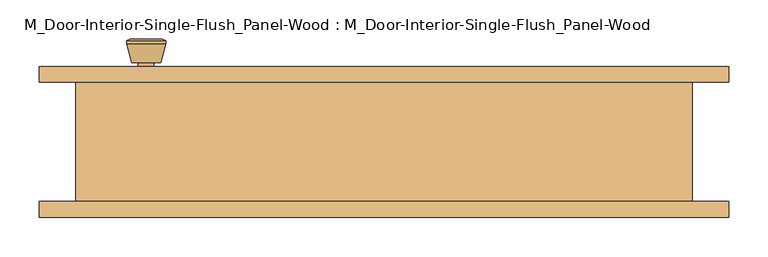
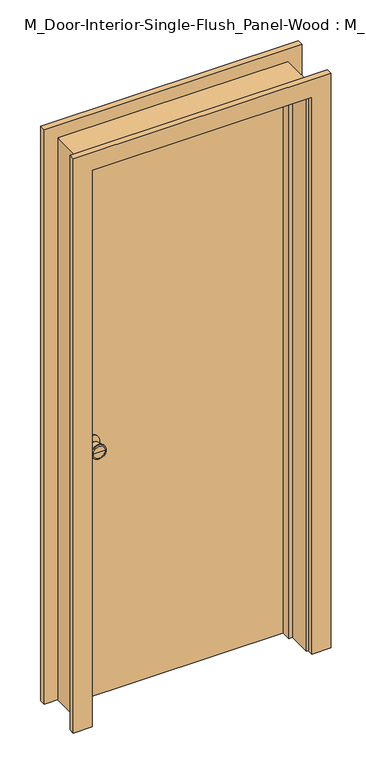
"""IFC4 building model written with IfcOpenShell, lengths in millimetres: door geometry, M_Door-Interior-Single-Flush_Panel-Wood : M_Door-Interior-Single-Flush_Panel-Wood."""

from ifc_helpers import new_model, si_unit, point, frame, frame_2d, origin, origin_with_axes, place, context, project, spatial, polyline, circle_curve, trimmed, segment, composite_curve, outline, extrude, faceted_brep, source, transform, mapped, element, save
from ifc_brep_helpers import plane_surface, cylinder_surface, revolved_surface, advanced_brep


def m_door_interior_single_flush_panel_wood_m_door_interior_da0777dc(model_context):
    return source(origin(), model_context, "Body", "SolidModel", [
        advanced_brep(
        [(-303.3, 32.025, 914.4), (-293.3, 32.025, 914.4), (-313.3, 32.025, 914.4), (-282.8241324, -16.975, 914.4), (-303.3, -16.975, 914.4), (-323.7758676, -16.975, 914.4), (-278.3, -15.1471319, 914.4), (-328.3, -15.1471319, 914.4), (-278.3, -11.6834537, 914.4), (-328.3, -11.6834537, 914.4), (-284.663764, 13.025, 914.4), (-321.936236, 13.025, 914.4), (-293.3, 13.025, 914.4), (-313.3, 13.025, 914.4)],
        [
            (0, 1),
            (1, 2, circle_curve(frame((-303.3, 32.025, 914.4), z_axis=(0.0, 1.0, 0.0), x_axis=(-1.0, 0.0, 0.0)), 10.0)),
            (2, 0),
            (2, 1, circle_curve(frame((-303.3, 32.025, 914.4), z_axis=(0.0, 1.0, 0.0), x_axis=(-1.0, 0.0, 0.0)), 10.0)),
            (3, 4),
            (4, 5),
            (5, 3, circle_curve(frame((-303.3, -16.975, 914.4), z_axis=(0.0, -1.0, 0.0), x_axis=(-1.0, 0.0, 0.0)), 20.4758676)),
            (3, 5, circle_curve(frame((-303.3, -16.975, 914.4), z_axis=(0.0, -1.0, 0.0), x_axis=(-1.0, 0.0, 0.0)), 20.4758676)),
            (6, 3),
            (5, 7),
            (7, 6, circle_curve(frame((-303.3, -15.1471319, 914.4), z_axis=(0.0, -1.0, 0.0), x_axis=(-1.0, 0.0, 0.0)), 25.0)),
            (6, 7, circle_curve(frame((-303.3, -15.1471319, 914.4), z_axis=(0.0, -1.0, 0.0), x_axis=(-1.0, 0.0, 0.0)), 25.0)),
            (8, 6),
            (7, 9),
            (9, 8, circle_curve(frame((-303.3, -11.6834537, 914.4), z_axis=(0.0, -1.0, 0.0), x_axis=(-1.0, 0.0, 0.0)), 25.0)),
            (8, 9, circle_curve(frame((-303.3, -11.6834537, 914.4), z_axis=(0.0, -1.0, 0.0), x_axis=(-1.0, 0.0, 0.0)), 25.0)),
            (10, 8),
            (9, 11),
            (11, 10, circle_curve(frame((-303.3, 13.025, 914.4), z_axis=(0.0, -1.0, 0.0), x_axis=(-1.0, 0.0, 0.0)), 18.636236)),
            (10, 11, circle_curve(frame((-303.3, 13.025, 914.4), z_axis=(0.0, -1.0, 0.0), x_axis=(-1.0, 0.0, 0.0)), 18.636236)),
            (12, 10),
            (11, 13),
            (13, 12, circle_curve(frame((-303.3, 13.025, 914.4), z_axis=(0.0, -1.0, 0.0), x_axis=(-1.0, 0.0, 0.0)), 10.0)),
            (12, 13, circle_curve(frame((-303.3, 13.025, 914.4), z_axis=(0.0, -1.0, 0.0), x_axis=(-1.0, 0.0, 0.0)), 10.0)),
            (1, 12),
            (13, 2),
        ],
        [
            plane_surface(frame((-303.3, 32.025, 914.4), z_axis=(0.0, 1.0, 0.0), x_axis=(-1.0, 0.0, 0.0))),
            plane_surface(frame((-303.3, -16.975, 914.4), z_axis=(0.0, -1.0, 0.0), x_axis=(-1.0, 0.0, 0.0))),
            revolved_surface(polyline([(-323.7758676, -16.975, 914.4), (-328.3, -15.1471319, 914.4)]), (-303.3, 32.025, 914.4), (0.0, 1.0, 0.0)),
            cylinder_surface(frame((-303.3, 32.025, 914.4), z_axis=(0.0, 1.0, 0.0), x_axis=(-1.0, 0.0, 0.0)), 25.0),
            revolved_surface(polyline([(-328.3, -11.6834537, 914.4), (-321.936236, 13.025, 914.4)]), (-303.3, 32.025, 914.4), (0.0, 1.0, 0.0)),
            plane_surface(frame((-303.3, 13.025, 914.4), z_axis=(0.0, 1.0, 0.0), x_axis=(-1.0, 0.0, 0.0))),
            cylinder_surface(frame((-303.3, 32.025, 914.4), z_axis=(0.0, 1.0, 0.0), x_axis=(-1.0, 0.0, 0.0)), 10.0),
        ],
        [
            (0, [[1, 2, 3]]),
            (0, [[-3, 4, -1]]),
            (1, [[5, 6, 7]]),
            (1, [[-6, -5, 8]]),
            (2, [[9, -7, 10, 11]]),
            (2, [[-10, -8, -9, 12]]),
            (3, [[13, -11, 14, 15]]),
            (3, [[-14, -12, -13, 16]]),
            (4, [[17, -15, 18, 19]]),
            (4, [[-18, -16, -17, 20]]),
            (5, [[21, -19, 22, 23]]),
            (5, [[-22, -20, -21, 24]]),
            (6, [[25, -23, 26, -2]]),
            (6, [[-26, -24, -25, -4]]),
        ],
    ),
        extrude(outline(composite_curve([segment(trimmed(circle_curve(frame_2d((914.4, -303.3)), 30.0), [point((914.4, -333.3))], [point((914.4, -273.3))], False, "CARTESIAN"), True, "CONTINUOUS"), segment(trimmed(circle_curve(frame_2d((914.4, -303.3)), 30.0), [point((914.4, -273.3))], [point((914.4, -333.3))], False, "CARTESIAN"), True, "CONTINUOUS")], self_intersect=False)), frame((0.0, 32.025, 0.0), z_axis=(0.0, 1.0, 0.0), x_axis=(0.0, 0.0, 1.0)), (0.0, 0.0, 1.0), 6.0),
        advanced_brep(
        [(-303.3, 79.025, 914.4), (-313.3, 79.025, 914.4), (-293.3, 79.025, 914.4), (-282.8241324, 128.025, 914.4), (-323.7758676, 128.025, 914.4), (-303.3, 128.025, 914.4), (-278.3, 126.1971319, 914.4), (-328.3, 126.1971319, 914.4), (-278.3, 122.7334537, 914.4), (-328.3, 122.7334537, 914.4), (-284.663764, 98.025, 914.4), (-321.936236, 98.025, 914.4), (-293.3, 98.025, 914.4), (-313.3, 98.025, 914.4)],
        [
            (0, 1),
            (1, 2, circle_curve(frame((-303.3, 79.025, 914.4), z_axis=(0.0, -1.0, 0.0), x_axis=(-1.0, 0.0, 0.0)), 10.0)),
            (2, 0),
            (2, 1, circle_curve(frame((-303.3, 79.025, 914.4), z_axis=(0.0, -1.0, 0.0), x_axis=(-1.0, 0.0, 0.0)), 10.0)),
            (3, 4, circle_curve(frame((-303.3, 128.025, 914.4), z_axis=(0.0, 1.0, 0.0), x_axis=(-1.0, 0.0, 0.0)), 20.4758676)),
            (4, 5),
            (5, 3),
            (4, 3, circle_curve(frame((-303.3, 128.025, 914.4), z_axis=(0.0, 1.0, 0.0), x_axis=(-1.0, 0.0, 0.0)), 20.4758676)),
            (6, 7, circle_curve(frame((-303.3, 126.1971319, 914.4), z_axis=(0.0, 1.0, 0.0), x_axis=(-1.0, 0.0, 0.0)), 25.0)),
            (7, 4),
            (3, 6),
            (7, 6, circle_curve(frame((-303.3, 126.1971319, 914.4), z_axis=(0.0, 1.0, 0.0), x_axis=(-1.0, 0.0, 0.0)), 25.0)),
            (8, 9, circle_curve(frame((-303.3, 122.7334537, 914.4), z_axis=(0.0, 1.0, 0.0), x_axis=(-1.0, 0.0, 0.0)), 25.0)),
            (9, 7),
            (6, 8),
            (9, 8, circle_curve(frame((-303.3, 122.7334537, 914.4), z_axis=(0.0, 1.0, 0.0), x_axis=(-1.0, 0.0, 0.0)), 25.0)),
            (10, 11, circle_curve(frame((-303.3, 98.025, 914.4), z_axis=(0.0, 1.0, 0.0), x_axis=(-1.0, 0.0, 0.0)), 18.636236)),
            (11, 9),
            (8, 10),
            (11, 10, circle_curve(frame((-303.3, 98.025, 914.4), z_axis=(0.0, 1.0, 0.0), x_axis=(-1.0, 0.0, 0.0)), 18.636236)),
            (12, 13, circle_curve(frame((-303.3, 98.025, 914.4), z_axis=(0.0, 1.0, 0.0), x_axis=(-1.0, 0.0, 0.0)), 10.0)),
            (13, 11),
            (10, 12),
            (13, 12, circle_curve(frame((-303.3, 98.025, 914.4), z_axis=(0.0, 1.0, 0.0), x_axis=(-1.0, 0.0, 0.0)), 10.0)),
            (1, 13),
            (12, 2),
        ],
        [
            plane_surface(frame((-303.3, 79.025, 914.4), z_axis=(0.0, -1.0, 0.0), x_axis=(-1.0, 0.0, 0.0))),
            plane_surface(frame((-303.3, 128.025, 914.4), z_axis=(0.0, 1.0, 0.0), x_axis=(-1.0, 0.0, 0.0))),
            revolved_surface(polyline([(-323.7758676, 128.025, 914.4), (-328.3, 126.1971319, 914.4)]), (-303.3, 79.025, 914.4), (0.0, -1.0, 0.0)),
            cylinder_surface(frame((-303.3, 79.025, 914.4), z_axis=(0.0, -1.0, 0.0), x_axis=(-1.0, 0.0, 0.0)), 25.0),
            revolved_surface(polyline([(-328.3, 122.7334537, 914.4), (-321.936236, 98.025, 914.4)]), (-303.3, 79.025, 914.4), (0.0, -1.0, 0.0)),
            plane_surface(frame((-303.3, 98.025, 914.4), z_axis=(0.0, -1.0, 0.0), x_axis=(-1.0, 0.0, 0.0))),
            cylinder_surface(frame((-303.3, 79.025, 914.4), z_axis=(0.0, -1.0, 0.0), x_axis=(-1.0, 0.0, 0.0)), 10.0),
        ],
        [
            (0, [[1, 2, 3]]),
            (0, [[-3, 4, -1]]),
            (1, [[5, 6, 7]]),
            (1, [[8, -7, -6]]),
            (2, [[9, 10, -5, 11]]),
            (2, [[12, -11, -8, -10]]),
            (3, [[13, 14, -9, 15]]),
            (3, [[16, -15, -12, -14]]),
            (4, [[17, 18, -13, 19]]),
            (4, [[20, -19, -16, -18]]),
            (5, [[21, 22, -17, 23]]),
            (5, [[24, -23, -20, -22]]),
            (6, [[-2, 25, -21, 26]]),
            (6, [[-4, -26, -24, -25]]),
        ],
    ),
        extrude(outline(composite_curve([segment(trimmed(circle_curve(frame_2d((914.4, -303.3)), 30.0), [point((914.4, -333.3))], [point((914.4, -273.3))], False, "CARTESIAN"), True, "CONTINUOUS"), segment(trimmed(circle_curve(frame_2d((914.4, -303.3)), 30.0), [point((914.4, -273.3))], [point((914.4, -333.3))], False, "CARTESIAN"), True, "CONTINUOUS")], self_intersect=False)), frame((0.0, 73.025, 0.0), z_axis=(0.0, 1.0, 0.0), x_axis=(0.0, 0.0, 1.0)), (0.0, 0.0, 1.0), 6.0),
        faceted_brep([(393.3, 73.025, 0.0), (393.3, -79.375, 0.0), (368.3, -79.375, 0.0), (368.3, 3.1, 0.0), (355.6, 3.1, 0.0), (355.6, 38.025, 0.0), (368.3, 38.025, 0.0), (368.3, 73.025, 0.0), (393.3, 73.025, 2025.0), (393.3, -79.375, 2025.0), (-393.3, -79.375, 2025.0), (-393.3, -79.375, 0.0), (-368.3, -79.375, 0.0), (-368.3, -79.375, 2000.0), (368.3, -79.375, 2000.0), (368.3, 3.1, 2000.0), (-368.3, 3.1, 2000.0), (-368.3, 3.1, 0.0), (-355.6, 3.1, 0.0), (-355.6, 3.1, 1987.3), (355.6, 3.1, 1987.3), (355.6, 38.025, 1987.3), (-355.6, 38.025, 1987.3), (-355.6, 38.025, 0.0), (-368.3, 38.025, 0.0), (-368.3, 38.025, 2000.0), (368.3, 38.025, 2000.0), (368.3, 73.025, 2000.0), (-368.3, 73.025, 2000.0), (-368.3, 73.025, 0.0), (-393.3, 73.025, 0.0), (-393.3, 73.025, 2025.0)], [[[0, 1, 2, 3, 4, 5, 6, 7]], [[1, 0, 8, 9]], [[2, 1, 9, 10, 11, 12, 13, 14]], [[3, 2, 14, 15]], [[4, 3, 15, 16, 17, 18, 19, 20]], [[5, 4, 20, 21]], [[6, 5, 21, 22, 23, 24, 25, 26]], [[7, 6, 26, 27]], [[0, 7, 27, 28, 29, 30, 31, 8]], [[9, 8, 31, 10]], [[15, 14, 13, 16]], [[21, 20, 19, 22]], [[27, 26, 25, 28]], [[30, 29, 24, 23, 18, 17, 12, 11]], [[10, 31, 30, 11]], [[16, 13, 12, 17]], [[22, 19, 18, 23]], [[28, 25, 24, 29]]]),
        extrude(outline(polyline([(368.3, 38.025), (-368.3, 38.025), (-368.3, 73.025), (368.3, 73.025), (368.3, 38.025)])), origin_with_axes(), (0.0, 0.0, 1.0), 2000.0),
        extrude(outline(polyline([(0.0, 374.65), (0.0, 439.65), (2071.35, 439.65), (2071.35, -439.65), (0.0, -439.65), (0.0, -374.65), (2006.35, -374.65), (2006.35, 374.65), (0.0, 374.65)])), frame((0.0, 73.025, 0.0), z_axis=(0.0, 1.0, 0.0), x_axis=(0.0, 0.0, 1.0)), (0.0, 0.0, 1.0), 20.0),
        extrude(outline(polyline([(0.0, 374.65), (0.0, 439.65), (2071.35, 439.65), (2071.35, -439.65), (0.0, -439.65), (0.0, -374.65), (2006.35, -374.65), (2006.35, 374.65), (0.0, 374.65)])), frame((0.0, -99.375, 0.0), z_axis=(0.0, 1.0, 0.0), x_axis=(0.0, 0.0, 1.0)), (0.0, 0.0, 1.0), 20.0),
    ])


if __name__ == "__main__":
    model = new_model("IFC4")
    model_context = context("Model", 3, world=origin())
    ifc_project = project(units=[si_unit("LENGTHUNIT", "METRE", prefix="MILLI")], contexts=[model_context])
    site = spatial("IfcSite", under=ifc_project)
    building = spatial("IfcBuilding", under=site)
    placement = place(None, origin())
    m_door_interior_single_flush_panel_wood_m_door_interior_shape = m_door_interior_single_flush_panel_wood_m_door_interior_da0777dc(model_context)
    element("IfcDoor", 1, ObjectType="M_Door-Interior-Single-Flush_Panel-Wood : M_Door-Interior-Single-Flush_Panel-Wood", at=placement, inside=building, context=model_context, shape_type="MappedRepresentation", body=[
        mapped(m_door_interior_single_flush_panel_wood_m_door_interior_shape, transform((0.0, 0.0, 0.0), x_axis=(1.0, 0.0, 0.0), y_axis=(0.0, 1.0, 0.0), z_axis=(0.0, 0.0, 1.0))),
    ])
    save(model, "model.ifc")

# Revit data of these elements
# Type "M_Door-Interior-Single-Flush_Panel-Wood : M_Door-Interior-Single-Flush_Panel-Wood"
#   Type Mark = "10"
#   Assembly Code = "C1020300"
#   Analytic Construction = "Wooden"
#   Thickness = 0' - 1.37795"
#   Thermal Resistance (R) = 2.5876 (h·ft²·°F)/BTU
#   Swing Angle [instance default] = 90.00°
#   Rough Width = 2' - 6.9685"
#   Rough Height = 6' - 7.72441"
#   Height = 6' - 6.74016"
#   Width = 2' - 5"
#   Heat Transfer Coefficient (U) = 0.3865 BTU/(h·ft²·°F)
#   Trim Material = Cherry
#   Panel Material = Cherry
#   Frame Material = Cherry
#   Door Handle Material = Aluminum
#   Visual Light Transmittance = 0
#   Solar Heat Gain Coefficient = 0
#   Wall Closure = (empty or 0)
#   Function = (empty or 0)
# Element 1 (IfcDoor, "M_Door-Interior-Single-Flush_Panel-Wood : M_Door-Interior-Single-Flush_Panel-Wood")
#   Materials on its faces: "Cherry", "Aluminum"
# Materials
#   "Cherry": class "Wood", colour RGB 226 177 128, transparency 0, Description = "Prunus Serotina", Cost = 0
#   "Aluminum": class "Metal", colour RGB 247 247 247, transparency 0, Description = "Aluminum 6061", Cost = 0
